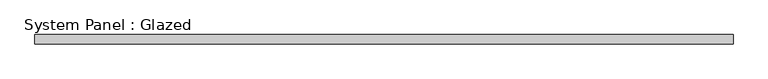
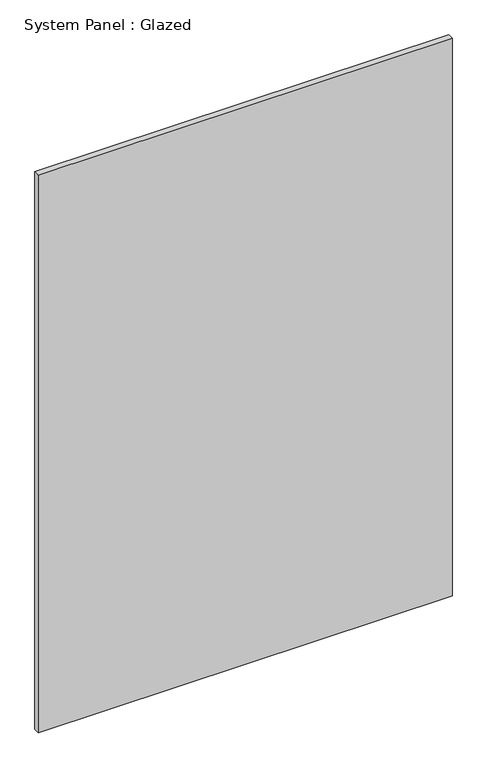
"""IFC4 building model written with IfcOpenShell, lengths in millimetres: plate geometry, System Panel : Glazed."""

from ifc_helpers import new_model, si_unit, origin, origin_with_axes, place, context, project, spatial, polyline, outline, extrude, source, transform, mapped, element, save


def system_panel_glazed_c01e4bb7(model_context):
    return source(origin(), model_context, "Body", "SweptSolid", [
        extrude(outline(polyline([(927.5, 24.5), (-927.5, 24.5), (-927.5, 49.5), (927.5, 49.5), (927.5, 24.5)])), origin_with_axes(), (0.0, 0.0, 1.0), 2643.2),
    ])


if __name__ == "__main__":
    model = new_model("IFC4")
    model_context = context("Model", 3, world=origin())
    ifc_project = project(units=[si_unit("LENGTHUNIT", "METRE", prefix="MILLI")], contexts=[model_context])
    site = spatial("IfcSite", under=ifc_project)
    building = spatial("IfcBuilding", under=site)
    placement = place(None, origin())
    system_panel_glazed_shape = system_panel_glazed_c01e4bb7(model_context)
    element("IfcPlate", 1, ObjectType="System Panel : Glazed", at=placement, inside=building, context=model_context, shape_type="MappedRepresentation", body=[
        mapped(system_panel_glazed_shape, transform((0.0, 0.0, 0.0), x_axis=(1.0, 0.0, 0.0), y_axis=(0.0, 1.0, 0.0), z_axis=(0.0, 0.0, 1.0))),
    ])
    save(model, "model.ifc")

# Revit data of these elements
# Type "System Panel : Glazed"
#   Construction Type Id = "GSP4R"
#   Analytic Construction = "1/8 in Pilkington single glazing"
#   Visual Light Transmittance = 0.9
#   Solar Heat Gain Coefficient = 0.86
#   Heat Transfer Coefficient (U) = 6.7069 W/(m²·K)
# Element 1 (IfcPlate, "System Panel : Glazed")
#   Materials on its faces: "Glass"
# Materials
#   "Glass": class "Glass", colour RGB 0 128 192, transparency 0.9, Description = "Soda Lime Glass", Cost = 0
